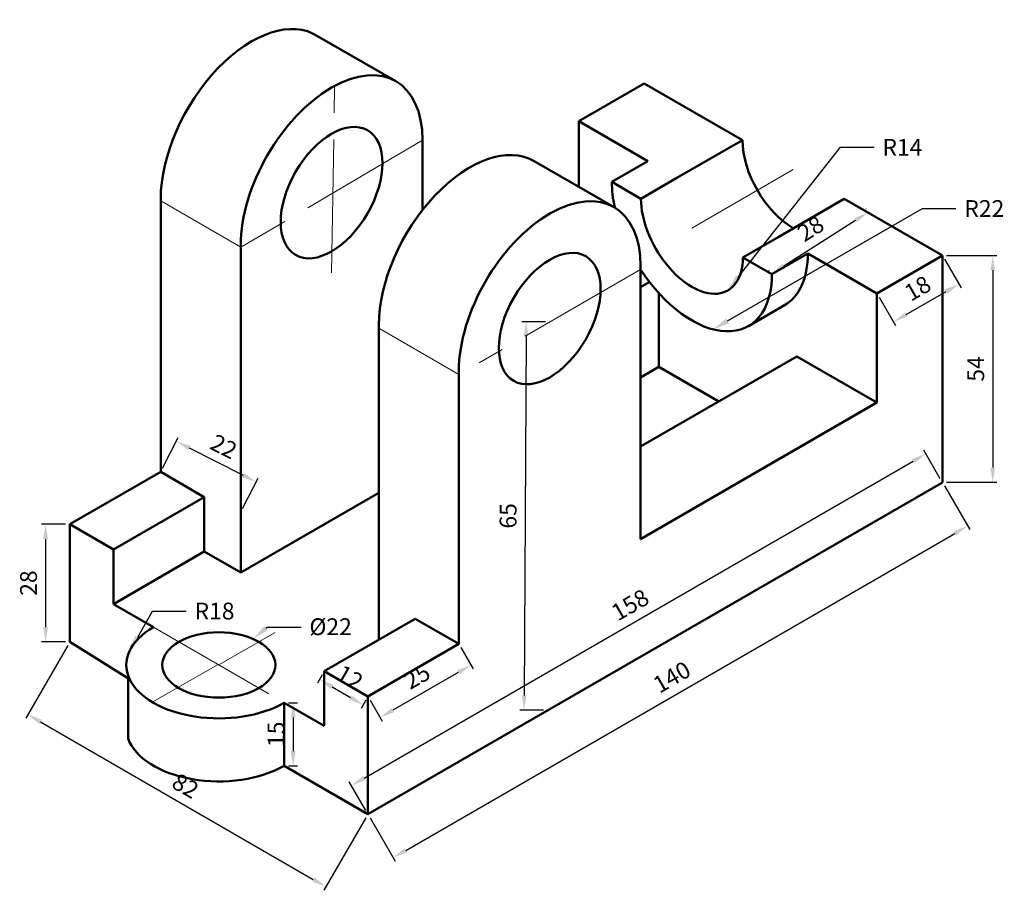
# Model space of a CAD drawing. Units: millimetres. Extents: x 2868 to 3103, y 662 to 870.
import ezdxf
from ezdxf import colors
from ezdxf.entities.mleader import LeaderData, LeaderLine
from ezdxf.math import Vec2, Vec3

# ---------------------------------------------------------------- set-up
doc = ezdxf.new("R2010")
doc.units = ezdxf.units.MM
doc.linetypes.add('CENTER', pattern=[50.8, 31.75, -6.35, 6.35, -6.35])
for name, color, linetype, lineweight in [('M-CNTR', 1, 'CENTER', 18), ('M-DIMS', 3, 'Continuous', 25), ('M-OUTL', 7, 'Continuous', 50), ('M-TEXT', 3, 'Continuous', 25)]:
    doc.layers.add(name, color=color, linetype=linetype, lineweight=lineweight)
doc.styles.get("Standard").update_dxf_attribs({"font": 'arial.ttf'})
doc.dimstyles.new('AM_ISO$0', dxfattribs={"dimtxt": 4, "dimasz": 3.5, "dimexe": 1, "dimexo": 1, "dimgap": 1.5, "dimtad": 1, "dimdsep": 46, "dimtxsty": 'Standard', "dimcen": 0, "dimclrd": 256, "dimclre": 256, "dimclrt": 2, "dimadec": 0, "dimazin": 2, "dimtp": 0.1, "dimtm": 0.1, "dimtfac": 0.71, "dimtmove": 0, "dimatfit": 3, "dimfxl": 1, "dimlwd": -1, "dimlwe": -1, "dimarcsym": 1})

# ---------------------------------------------------------------- blocks, each defined once
blk = doc.blocks.new('*D3')
at = {"layer": 'Defpoints', "color": 0, "transparency": 16777216}
for p in [(3088.17, 759.61), (3094.17, 749.21), (2951.34, 680.61)]:
    blk.add_point(p, dxfattribs=at)
at = {"layer": 'M-DIMS', "color": 0, "linetype": 'ByBlock', "transparency": 16777216}
for p, q in [((3088.67, 758.74), (3094.67, 748.35)), ((2960.37, 671.96), (3091.14, 747.46)), ((2951.84, 679.74), (2957.84, 669.35))]:
    blk.add_line(p, q, dxfattribs=at)
at = {"layer": 'M-DIMS', "color": 0, "transparency": 16777216}
for points in [[(3090.84, 747.97), (3091.43, 746.96), (3094.17, 749.21)], [(2960.07, 672.47), (2960.66, 671.46), (2957.34, 670.21)]]:
    blk.add_solid(points, dxfattribs=at)
at = {"layer": 'M-DIMS', "color": 0, "transparency": 16777216, "insert": (3023.98, 712.78), "char_height": 4, "attachment_point": 5, "rotation": 30}
blk.add_mtext('140', dxfattribs=at)
blk = doc.blocks.new('*D4')
at = {"layer": 'Defpoints', "color": 0, "transparency": 16777216}
for p in [(3088.17, 813.61), (3088.17, 759.61), (3100.17, 759.61)]:
    blk.add_point(p, dxfattribs=at)
at = {"layer": 'M-DIMS', "color": 0, "linetype": 'ByBlock', "transparency": 16777216}
for p, q in [((3089.17, 813.61), (3101.17, 813.61)), ((3100.17, 810.11), (3100.17, 763.11)), ((3089.17, 759.61), (3101.17, 759.61))]:
    blk.add_line(p, q, dxfattribs=at)
at = {"layer": 'M-DIMS', "color": 0, "transparency": 16777216}
for points in [[(3099.58, 810.11), (3100.75, 810.11), (3100.17, 813.61)], [(3099.58, 763.11), (3100.75, 763.11), (3100.17, 759.61)]]:
    blk.add_solid(points, dxfattribs=at)
at = {"layer": 'M-DIMS', "color": 0, "transparency": 16777216, "insert": (3096.63, 786.61), "char_height": 4, "attachment_point": 5, "rotation": 90}
blk.add_mtext('54', dxfattribs=at)
blk = doc.blocks.new('*D5')
at = {"layer": 'Defpoints', "color": 0, "transparency": 16777216}
for p in [(3070.45, 823.92), (3070.54, 823.79), (3047.55, 809.16)]:
    blk.add_point(p, dxfattribs=at)
at = {"layer": 'M-DIMS', "color": 0, "linetype": 'ByBlock', "transparency": 16777216}
for p, q in [((3070, 824.63), (3069.91, 824.76)), ((3050.42, 811.17), (3067.5, 822.04)), ((3047.01, 810), (3046.93, 810.13))]:
    blk.add_line(p, q, dxfattribs=at)
at = {"layer": 'M-DIMS', "color": 0, "transparency": 16777216}
for points in [[(3067.18, 822.53), (3067.81, 821.55), (3070.45, 823.92)], [(3050.11, 811.66), (3050.73, 810.68), (3047.47, 809.29)]]:
    blk.add_solid(points, dxfattribs=at)
at = {"layer": 'M-DIMS', "color": 0, "transparency": 16777216, "insert": (3057.06, 819.59), "char_height": 4, "attachment_point": 5, "rotation": 32.4771}
blk.add_mtext('28', dxfattribs=at)
blk = doc.blocks.new('*D6')
at = {"layer": 'Defpoints', "color": 0, "transparency": 16777216}
for p in [(3088.17, 813.61), (3092.1, 806.8), (3072.58, 804.61)]:
    blk.add_point(p, dxfattribs=at)
at = {"layer": 'M-DIMS', "color": 0, "linetype": 'ByBlock', "transparency": 16777216}
for p, q in [((3088.67, 812.74), (3092.6, 805.94)), ((3079.54, 799.55), (3089.06, 805.05)), ((3073.08, 803.74), (3077.01, 796.94))]:
    blk.add_line(p, q, dxfattribs=at)
at = {"layer": 'M-DIMS', "color": 0, "transparency": 16777216}
for points in [[(3088.77, 805.56), (3089.36, 804.55), (3092.1, 806.8)], [(3079.25, 800.06), (3079.83, 799.05), (3076.51, 797.8)]]:
    blk.add_solid(points, dxfattribs=at)
at = {"layer": 'M-DIMS', "color": 0, "transparency": 16777216, "insert": (3082.53, 805.37), "char_height": 4, "attachment_point": 5, "rotation": 30}
blk.add_mtext('18', dxfattribs=at)
blk = doc.blocks.new('*D7')
at = {"layer": 'Defpoints', "color": 0, "transparency": 16777216}
for p in [(2880.32, 749.61), (2874.55, 721.61), (2880.32, 721.61)]:
    blk.add_point(p, dxfattribs=at)
at = {"layer": 'M-DIMS', "color": 0, "linetype": 'ByBlock', "transparency": 16777216}
for p, q in [((2879.32, 749.61), (2873.55, 749.61)), ((2874.55, 746.11), (2874.55, 725.11)), ((2879.32, 721.61), (2873.55, 721.61))]:
    blk.add_line(p, q, dxfattribs=at)
at = {"layer": 'M-DIMS', "color": 0, "transparency": 16777216}
for points in [[(2873.97, 746.11), (2875.14, 746.11), (2874.55, 749.61)], [(2873.97, 725.11), (2875.14, 725.11), (2874.55, 721.61)]]:
    blk.add_solid(points, dxfattribs=at)
at = {"layer": 'M-DIMS', "color": 0, "transparency": 16777216, "insert": (2871.01, 735.61), "char_height": 4, "attachment_point": 5, "rotation": 90}
blk.add_mtext('28', dxfattribs=at)
blk = doc.blocks.new('*D8')
at = {"layer": 'Defpoints', "color": 0, "transparency": 16777216}
for p in [(2880.32, 721.61), (2951.34, 680.61), (2941.35, 663.31)]:
    blk.add_point(p, dxfattribs=at)
at = {"layer": 'M-DIMS', "color": 0, "linetype": 'ByBlock', "transparency": 16777216}
for p, q in [((2879.82, 720.74), (2869.84, 703.45)), ((2873.37, 702.56), (2938.32, 665.06)), ((2950.84, 679.74), (2940.85, 662.45))]:
    blk.add_line(p, q, dxfattribs=at)
at = {"layer": 'M-DIMS', "color": 0, "transparency": 16777216}
for points in [[(2873.66, 703.07), (2873.08, 702.06), (2870.34, 704.31)], [(2938.61, 665.57), (2938.03, 664.56), (2941.35, 663.31)]]:
    blk.add_solid(points, dxfattribs=at)
at = {"layer": 'M-DIMS', "color": 0, "transparency": 16777216, "insert": (2907.62, 686.88), "char_height": 4, "attachment_point": 5, "rotation": 330}
blk.add_mtext('82', dxfattribs=at)
blk = doc.blocks.new('*D9')
at = {"layer": 'Defpoints', "color": 0, "transparency": 16777216}
for p in [(2940.94, 714.61), (2951.34, 708.61), (2950.2, 706.64)]:
    blk.add_point(p, dxfattribs=at)
at = {"layer": 'M-DIMS', "color": 0, "linetype": 'ByBlock', "transparency": 16777216}
for p, q in [((2940.44, 713.74), (2939.31, 711.77)), ((2942.84, 710.89), (2947.17, 708.39)), ((2950.84, 707.74), (2949.7, 705.77))]:
    blk.add_line(p, q, dxfattribs=at)
at = {"layer": 'M-DIMS', "color": 0, "transparency": 16777216}
for points in [[(2943.13, 711.39), (2942.54, 710.38), (2939.81, 712.64)], [(2947.46, 708.89), (2946.87, 707.88), (2950.2, 706.64)]]:
    blk.add_solid(points, dxfattribs=at)
at = {"layer": 'M-DIMS', "color": 0, "transparency": 16777216, "insert": (2946.76, 712.67), "char_height": 4, "attachment_point": 5, "rotation": 330}
blk.add_mtext('12', dxfattribs=at)
blk = doc.blocks.new('*D10')
at = {"layer": 'Defpoints', "color": 0, "transparency": 16777216}
for p in [(2972.99, 721.11), (2951.34, 708.61), (2954.23, 703.6)]:
    blk.add_point(p, dxfattribs=at)
at = {"layer": 'M-DIMS', "color": 0, "linetype": 'ByBlock', "transparency": 16777216}
for p, q in [((2973.49, 720.24), (2976.38, 715.23)), ((2972.85, 714.35), (2957.26, 705.35)), ((2951.84, 707.74), (2954.73, 702.73))]:
    blk.add_line(p, q, dxfattribs=at)
at = {"layer": 'M-DIMS', "color": 0, "transparency": 16777216}
for points in [[(2972.55, 714.85), (2973.14, 713.84), (2975.88, 716.1)], [(2956.97, 705.85), (2957.55, 704.84), (2954.23, 703.6)]]:
    blk.add_solid(points, dxfattribs=at)
at = {"layer": 'M-DIMS', "color": 0, "transparency": 16777216, "insert": (2963.28, 712.92), "char_height": 4, "attachment_point": 5, "rotation": 30}
blk.add_mtext('25', dxfattribs=at)
blk = doc.blocks.new('*D11')
at = {"layer": 'Defpoints', "color": 0, "transparency": 16777216}
for p in [(2994.63, 797.82), (2988.54, 705.35), (2994.14, 705.32)]:
    blk.add_point(p, dxfattribs=at)
at = {"layer": 'M-DIMS', "color": 0, "linetype": 'ByBlock', "transparency": 16777216}
for p, q in [((2993.63, 797.82), (2988.03, 797.85)), ((2989.01, 794.35), (2988.56, 708.85)), ((2993.14, 705.33), (2987.54, 705.36))]:
    blk.add_line(p, q, dxfattribs=at)
at = {"layer": 'M-DIMS', "color": 0, "transparency": 16777216}
for points in [[(2988.43, 794.35), (2989.59, 794.34), (2989.03, 797.85)], [(2987.97, 708.85), (2989.14, 708.85), (2988.54, 705.35)]]:
    blk.add_solid(points, dxfattribs=at)
at = {"layer": 'M-DIMS', "color": 0, "transparency": 16777216, "insert": (2985.24, 751.62), "char_height": 4, "attachment_point": 5, "rotation": 89.6953}
blk.add_mtext('65', dxfattribs=at)
blk = doc.blocks.new('*D12')
at = {"layer": 'Defpoints', "color": 0, "transparency": 16777216}
for p in [(2931.42, 707.11), (2931.42, 692.11), (2933.52, 692.11)]:
    blk.add_point(p, dxfattribs=at)
at = {"layer": 'M-DIMS', "color": 0, "linetype": 'ByBlock', "transparency": 16777216}
for p, q in [((2932.42, 707.11), (2934.52, 707.11)), ((2933.52, 703.61), (2933.52, 695.61)), ((2932.42, 692.11), (2934.52, 692.11))]:
    blk.add_line(p, q, dxfattribs=at)
at = {"layer": 'M-DIMS', "color": 0, "transparency": 16777216}
for points in [[(2932.94, 703.61), (2934.11, 703.61), (2933.52, 707.11)], [(2932.94, 695.61), (2934.11, 695.61), (2933.52, 692.11)]]:
    blk.add_solid(points, dxfattribs=at)
at = {"layer": 'M-DIMS', "color": 0, "transparency": 16777216, "insert": (2929.98, 699.61), "char_height": 4, "attachment_point": 5, "rotation": 90}
blk.add_mtext('15', dxfattribs=at)
blk = doc.blocks.new('*D13')
at = {"layer": 'Defpoints', "color": 0, "transparency": 16777216}
for p in [(2901.97, 762.11), (2924.71, 759.72), (2921.02, 752.44)]:
    blk.add_point(p, dxfattribs=at)
at = {"layer": 'M-DIMS', "color": 0, "linetype": 'ByBlock', "transparency": 16777216}
for p, q in [((2902.42, 763), (2906.11, 770.27)), ((2908.78, 767.8), (2921.59, 761.3)), ((2921.48, 753.34), (2925.17, 760.61))]:
    blk.add_line(p, q, dxfattribs=at)
at = {"layer": 'M-DIMS', "color": 0, "transparency": 16777216}
for points in [[(2909.05, 768.32), (2908.52, 767.28), (2905.66, 769.38)], [(2921.86, 761.82), (2921.33, 760.78), (2924.71, 759.72)]]:
    blk.add_solid(points, dxfattribs=at)
at = {"layer": 'M-DIMS', "color": 0, "transparency": 16777216, "insert": (2916.77, 767.68), "char_height": 4, "attachment_point": 5, "rotation": 333.1053}
blk.add_mtext('22', dxfattribs=at)
blk = doc.blocks.new('*D14')
at = {"layer": 'Defpoints', "color": 0, "transparency": 16777216}
for p in [(3084.24, 766.42), (3088.17, 759.61), (2951.34, 680.61)]:
    blk.add_point(p, dxfattribs=at)
at = {"layer": 'M-DIMS', "linetype": 'ByBlock', "transparency": 16777216}
for p, q in [((3087.67, 760.47), (3083.74, 767.28)), ((2950.43, 689.17), (3081.2, 764.67)), ((2950.84, 681.47), (2946.9, 688.28))]:
    blk.add_line(p, q, dxfattribs=at)
at = {"layer": 'M-DIMS', "transparency": 16777216}
for points in [[(3080.91, 765.17), (3081.5, 764.16), (3084.24, 766.42)], [(2950.14, 689.67), (2950.73, 688.66), (2947.4, 687.42)]]:
    blk.add_solid(points, dxfattribs=at)
at = {"layer": 'M-DIMS', "color": 2, "transparency": 16777216, "insert": (3014.05, 729.99), "char_height": 4, "attachment_point": 5, "rotation": 30}
blk.add_mtext('158', dxfattribs=at)

msp = doc.modelspace()

# ---------------------------------------------------------------- linework, layer by layer
at = {"layer": 'M-CNTR'}
for p, q in [((2942.675, 809.493), (2943.379, 854.001)), ((2964.326, 841.107), (2930.558, 821.143)), ((3052.66, 834.107), (3028.499, 820.158)), ((2921.025, 815.639), (2901.972, 826.639)), ((2930.558, 821.143), (2921.025, 815.639)), ((3016.287, 810.321), (2972.986, 785.321)), ((2972.986, 785.321), (2953.933, 796.321)), ((2900.24, 725.107), (2931.417, 707.107)), ((2915.828, 716.107), (2929.263, 723.864)), ((2915.686, 716.189), (2899.936, 707.286))]:
    msp.add_line(p, q, dxfattribs=at)
at = {"layer": 'M-OUTL'}
for p, q in [((2939.343, 865.873), (2957.98, 855.126)), ((3017.153, 854.607), (3001.565, 845.607)), ((3017.153, 854.607), (3040.536, 841.107)), ((3018.019, 836.107), (3001.565, 845.607)), ((3001.565, 845.607), (3001.565, 829.963)), ((2964.326, 841.107), (2964.326, 824.461)), ((3024.948, 832.107), (3040.536, 841.107)), ((2990.893, 836.124), (3009.946, 825.124)), ((3018.019, 836.107), (3009.446, 831.158)), ((3009.446, 831.158), (3016.374, 827.158)), ((3024.948, 832.107), (3016.374, 827.158)), ((2901.972, 762.107), (2901.972, 827.107)), ((3049.196, 818.107), (3064.785, 827.107)), ((3064.785, 827.107), (3088.167, 813.607)), ((3049.196, 818.107), (3040.623, 813.158)), ((2921.025, 738.107), (2921.025, 816.107)), ((3056.124, 814.107), (3047.551, 809.158)), ((3072.579, 804.607), (3056.124, 814.107)), ((3040.623, 813.158), (3047.551, 809.158)), ((3072.579, 804.607), (3088.167, 813.607)), ((3088.167, 813.607), (3088.167, 759.607)), ((3016.287, 746.107), (3016.287, 811.107)), ((3016.287, 806.107), (3018.316, 807.279)), ((3020.617, 787.107), (3020.617, 804.532)), ((3072.579, 778.607), (3072.579, 804.607)), ((3072.579, 778.607), (3072.579, 804.607)), ((3050.544, 801.773), (3041.971, 796.823)), ((2953.933, 797.107), (2953.933, 732.107)), ((3053.526, 789.607), (3016.287, 768.107)), ((3072.579, 778.607), (3053.526, 789.607)), ((2972.986, 721.107), (2972.986, 786.107)), ((3016.287, 784.607), (3020.617, 787.107)), ((3034.907, 778.857), (3020.617, 787.107)), ((3016.287, 746.107), (3072.579, 778.607)), ((3056.991, 769.607), (3016.287, 746.107)), ((2901.972, 762.107), (2880.321, 749.607)), ((2880.321, 749.607), (2901.972, 762.107)), ((2901.972, 762.107), (2912.364, 756.107)), ((2951.335, 680.607), (3088.167, 759.607)), ((2912.364, 756.107), (2890.714, 743.607)), ((2912.364, 743.107), (2912.364, 756.107)), ((2921.025, 738.107), (2953.933, 757.107)), ((2880.321, 736.607), (2880.321, 749.607)), ((2890.714, 743.607), (2880.321, 749.607)), ((2880.321, 749.607), (2880.321, 721.607)), ((2890.714, 730.607), (2890.714, 743.607)), ((2890.714, 730.607), (2912.364, 743.107)), ((2912.364, 743.107), (2921.025, 738.107)), ((2953.933, 732.107), (2953.933, 722.107)), ((2900.24, 725.107), (2890.714, 730.607)), ((2962.594, 727.107), (2940.943, 714.607)), ((2972.986, 721.107), (2962.594, 727.107)), ((2880.321, 721.607), (2894.558, 712.763)), ((2951.335, 708.607), (2972.986, 721.107)), ((2894.221, 713.582), (2894.221, 698.582)), ((2940.943, 714.607), (2951.335, 708.607)), ((2940.943, 714.607), (2940.943, 701.607)), ((2951.335, 680.607), (2951.335, 708.607)), ((2931.417, 707.107), (2931.417, 692.107)), ((2931.417, 707.107), (2940.943, 701.607)), ((2931.417, 692.107), (2951.335, 680.607))]:
    msp.add_line(p, q, dxfattribs=at)
for centre, major_axis, start_param, end_param in [((2923.623, 839.607), (-15.309, -26.517), 3.1143616, 5.4977871), ((2942.675, 828.607), (-15.309, -26.517), 2.3561945, 5.4977871), ((2975.584, 809.607), (-15.309, -26.517), 3.1415927, 5.4977871), ((3052.66, 834.107), (8.573, -14.849), 3.9269908, 5.4977871), ((3028.499, 820.158), (13.472, -23.335), 3.9269908, 4.1912918), ((2994.637, 798.607), (-15.309, -26.517), 2.3561945, 5.4977871), ((3028.499, 820.158), (8.573, -14.849), 3.9269908, 7.0685835), ((3037.072, 825.107), (13.472, -23.335), 6.2831853, 7.0685835), ((3028.499, 820.158), (13.472, -23.335), 4.8020753, 7.0685835), ((2915.828, 716.107), (-22.045, 0), 5.4977871, 8.6393798), ((2915.828, 701.107), (-22.045, 0), 6.4828979, 8.6393798)]:
    msp.add_ellipse(centre, major_axis=major_axis, ratio=0.5773503, start_param=start_param, end_param=end_param, dxfattribs=at)
for centre, major_axis in [((2942.675, 828.607), (-8.573, -14.849)), ((2994.637, 798.607), (-8.573, -14.849)), ((2915.828, 716.107), (-13.472, 0))]:
    msp.add_ellipse(centre, major_axis=major_axis, ratio=0.5773503, dxfattribs=at)

# ---------------------------------------------------------------- dimensions: what is measured, and where the dimension line sits
at = {"layer": 'M-DIMS'}
for p1, p2, distance, text, picture, middle in [((3047.551, 809.158), (3070.535, 823.787), 0.158, '28', '*D5', (3057.056, 819.594)), ((2994.632, 797.818), (2994.141, 705.321), -5.603, '65', '*D11', (2985.242, 751.618)), ((2901.972, 762.107), (2921.025, 752.444), 8.155, '22', '*D13', (2916.774, 767.677)), ((2951.335, 680.607), (3088.167, 759.607), -12, '140', '*D3', (3023.98, 712.783))]:
    dim = msp.add_aligned_dim(p1=p1, p2=p2, distance=distance, text=text, dimstyle='AM_ISO$0', override={"dimpost": '', "dimclrd": 0, "dimclre": 0, "dimclrt": 0}, dxfattribs=at)
    dim.commit()
    dim.dimension.update_dxf_attribs({"geometry": picture, "text_midpoint": middle})
for p1, p2, distance, override, picture, middle in [((3072.579, 804.607), (3088.167, 813.607), -7.856, {"dimpost": '', "dimclrd": 0, "dimclre": 0, "dimclrt": 0}, '*D6', (3082.53, 805.371)), ((3088.167, 813.607), (3088.167, 759.607), 12, {"dimclrd": 0, "dimclre": 0, "dimclrt": 0}, '*D4', (3096.633, 786.607)), ((2880.321, 749.607), (2880.321, 721.607), -5.767, {"dimclrd": 0, "dimclre": 0, "dimclrt": 0}, '*D7', (2871.013, 735.607)), ((2880.321, 721.607), (2951.335, 680.607), -19.969, {"dimclrd": 0, "dimclre": 0, "dimclrt": 0}, '*D8', (2907.615, 686.881)), ((2972.986, 721.107), (2951.335, 708.607), 5.783, {"dimclrd": 0, "dimclre": 0, "dimclrt": 0}, '*D10', (2963.281, 712.917)), ((2940.943, 714.607), (2951.335, 708.607), -2.276, {"dimclrd": 0, "dimclre": 0, "dimclrt": 0}, '*D9', (2946.756, 712.675)), ((2931.417, 707.107), (2931.417, 692.107), 2.105, {"dimpost": '', "dimclrd": 0, "dimclre": 0, "dimclrt": 0}, '*D12', (2929.979, 699.607))]:
    dim = msp.add_aligned_dim(p1=p1, p2=p2, distance=distance, dimstyle='AM_ISO$0', override=override, dxfattribs=at)
    dim.commit()
    dim.dimension.update_dxf_attribs({"geometry": picture, "text_midpoint": middle})
dim = msp.add_linear_dim(base=(3084.236, 766.417), p1=(2951.335, 680.607), p2=(3088.167, 759.607), angle=30, dimstyle='AM_ISO$0', override={"dimrnd": 0}, dxfattribs=at)
dim.commit()
dim.dimension.update_dxf_attribs({"geometry": '*D14', "text_midpoint": (3014.049, 729.985)})

# ---------------------------------------------------------------- leaders
at = {"layer": 'M-TEXT'}
ml = msp.add_multileader_mtext('Standard', dxfattribs=at)
ml.set_content('{\\C2;R14}', color=256)
ml.set_leader_properties()
ml.build(insert=Vec2(0, 0))
ctx = ml.context
ctx.base_point, ctx.plane_origin = Vec3(3071.882, 839.406), Vec3(3037.072, 805.308)
notes = []
notes.append((ctx, [(0, (1, 1, 0), (3063.882, 839.406), (1, 0), 8, [(0, [(3037.072, 805.308)], 0, [])])]))
ctx.mtext.insert, ctx.mtext.flow_direction = Vec3(3073.882, 841.406), 5
ml = msp.add_multileader_mtext('Standard', dxfattribs=at)
ml.set_content('{\\C2;R22}', color=256)
ml.set_leader_properties()
ml.build(insert=Vec2(0, 0))
ctx = ml.context
ctx.base_point, ctx.plane_origin = Vec3(3091.39, 824.816), Vec3(3033.535, 796.032)
notes.append((ctx, [(0, (1, 1, 0), (3083.39, 824.816), (1, 0), 8, [(0, [(3033.535, 796.032)], 0, [])])]))
ctx.mtext.insert, ctx.mtext.flow_direction = Vec3(3093.39, 826.816), 5
ml = msp.add_multileader_mtext('Standard', dxfattribs=at)
ml.set_content('{\\C2;R18}', color=256)
ml.set_leader_properties()
ml.build(insert=Vec2(0, 0))
ctx = ml.context
ctx.base_point, ctx.plane_origin = Vec3(2908.04, 728.919), Vec3(2894.49, 719.305)
notes.append((ctx, [(0, (1, 1, 0), (2900.04, 728.919), (1, 0), 8, [(0, [(2894.49, 719.305)], 0, [])])]))
ctx.mtext.insert, ctx.mtext.flow_direction = Vec3(2910.04, 730.953), 5
ml = msp.add_multileader_mtext('Standard', dxfattribs=at)
ml.set_content('{\\C2;%%C22}', color=256)
ml.set_leader_properties()
ml.build(insert=Vec2(0, 0))
ctx = ml.context
ctx.base_point, ctx.plane_origin = Vec3(2935.396, 725.143), Vec3(2923.93, 722.322)
notes.append((ctx, [(0, (1, 1, 0), (2927.396, 725.143), (1, 0), 8, [(0, [(2923.93, 722.322)], 0, [])])]))
ctx.mtext.insert, ctx.mtext.flow_direction = Vec3(2937.396, 727.223), 5
for ctx, leaders in notes:
    for number, flags, end, landing, length, lines in leaders:
        leader = LeaderData()
        leader.index, (leader.has_last_leader_line, leader.has_dogleg_vector, leader.attachment_direction) = number, flags
        leader.last_leader_point, leader.dogleg_vector, leader.dogleg_length = Vec3(end), Vec3(landing), length
        for number, points, colour, breaks in lines:
            line = LeaderLine()
            line.index, line.vertices, line.color, line.breaks = number, Vec3.list(points), colors.encode_raw_color(colour), breaks
            leader.lines.append(line)
        ctx.leaders.append(leader)

doc.saveas('drawing.dxf')
